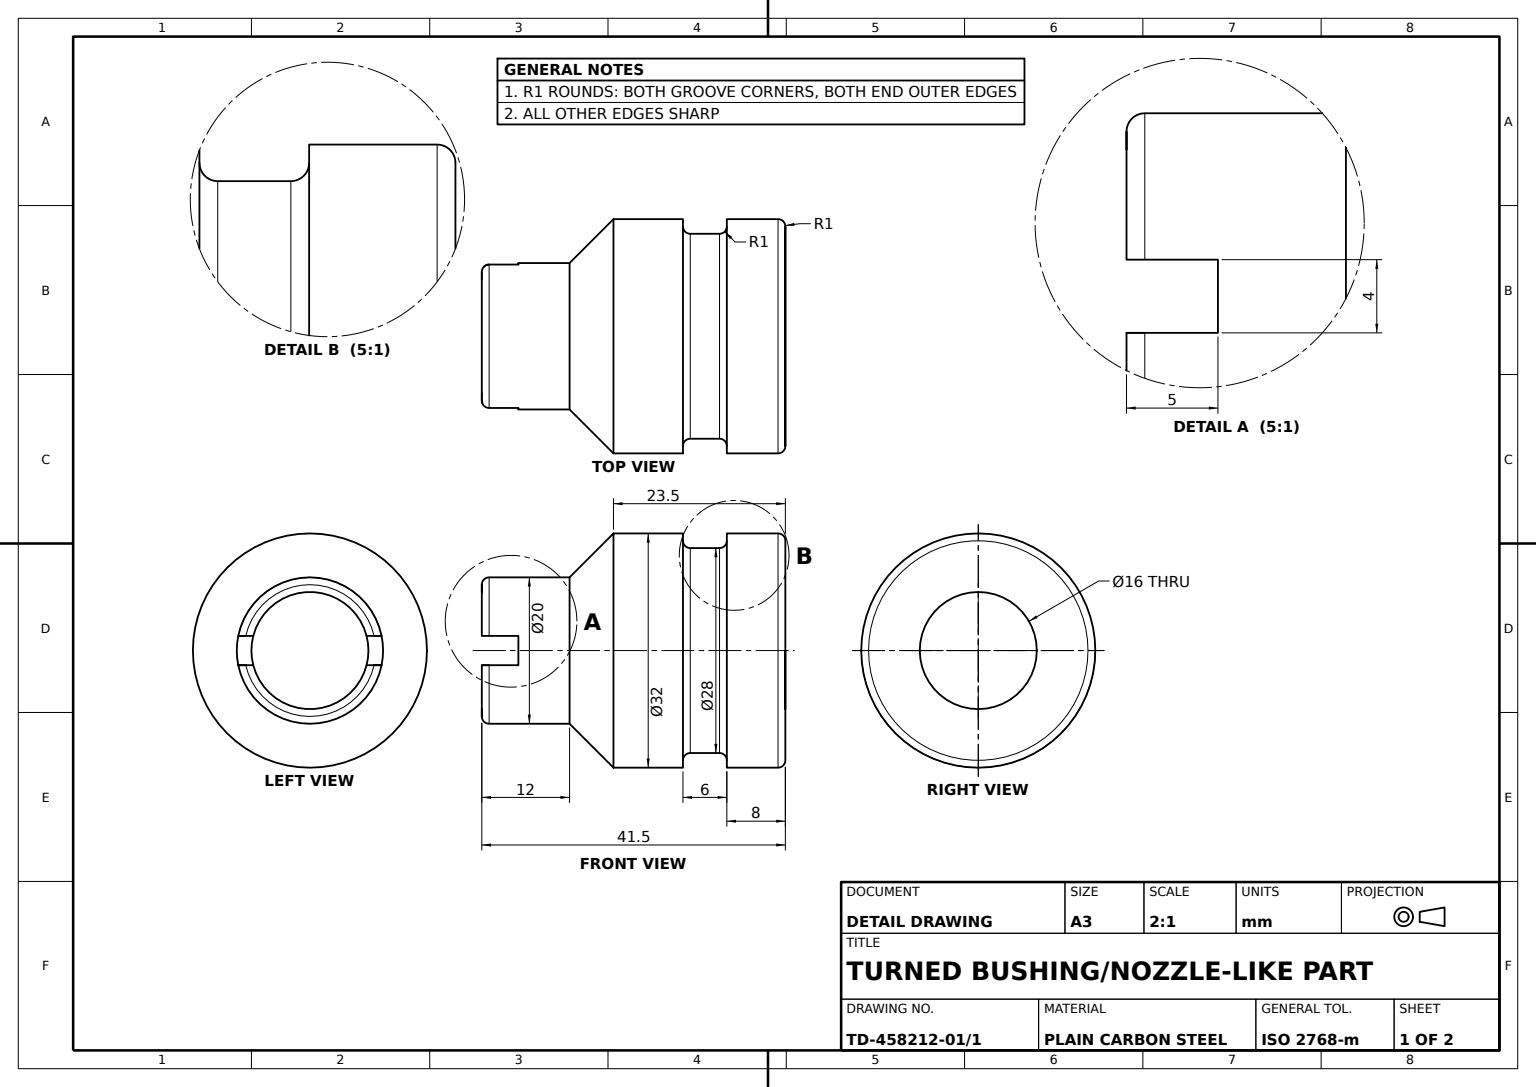
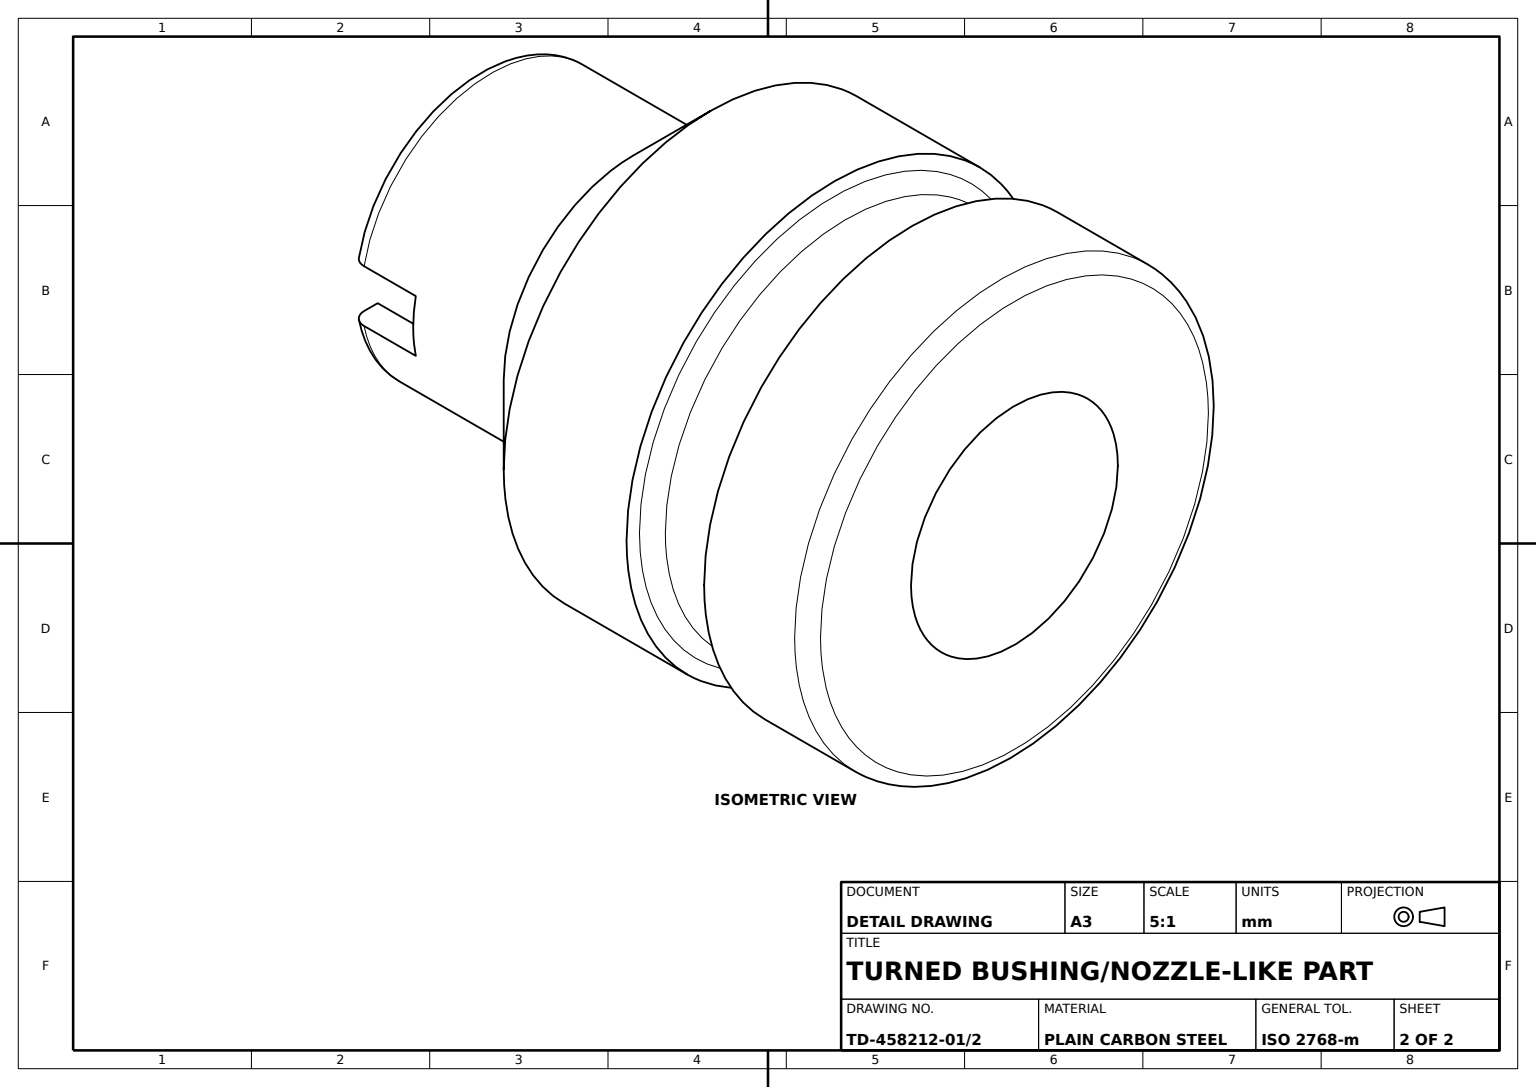
from build123d import *

# Parameters (mm, degrees)
END_SLOT_CUT_DEPTH      = 51.539588475
END_SLOT_CUT_DEPTH_BACK = 51.539588475
END_SLOT_PROFILE_W      = 5
END_SLOT_PROFILE_H      = 4


with BuildPart() as part:
    # Bushing Revolve Profile → Stepped Bushing Body (revolve)
    with BuildSketch(Plane.XY, mode=Mode.PRIVATE) as stepped_bushing_body_sk:
        with BuildLine():
            Line((0, 0), (0, -1))
            ThreePointArc((0, -1), (0.292893219, -1.707106781), (1, -2))
            Line((1, -2), (12, -2))
            Line((12, -2), (18, -8))
            Line((18, -8), (27.5, -8))
            Line((27.5, -8), (27.5, -7))
            ThreePointArc((27.5, -7), (27.792893219, -6.292893219), (28.5, -6))
            Line((28.5, -6), (32.5, -6))
            ThreePointArc((32.5, -6), (33.207106781, -6.292893219), (33.5, -7))
            Line((33.5, -7), (33.5, -8))
            Line((33.5, -8), (40.5, -8))
            ThreePointArc((40.5, -8), (41.207106781, -7.707106781), (41.5, -7))
            Line((41.5, -7), (41.5, 0))
            Line((41.5, 0), (0, 0))
        make_face()
    revolve(stepped_bushing_body_sk.sketch.rotate(Axis((-18.754371045, 8, 0), (1, 0, 0)), 270), axis=Axis((-18.754371045, 8, 0), (1, 0, 0)))

    # End Slot Profile → End Slot Cut (cut, two sides: drawn at the far end of the back side and taken through both)
    with BuildSketch(Plane.XY.offset(-END_SLOT_CUT_DEPTH_BACK)):
        with Locations((2.5, 8)):
            Rectangle(END_SLOT_PROFILE_W, END_SLOT_PROFILE_H)
    extrude(amount=END_SLOT_CUT_DEPTH + END_SLOT_CUT_DEPTH_BACK, mode=Mode.SUBTRACT)


solid = part.part
